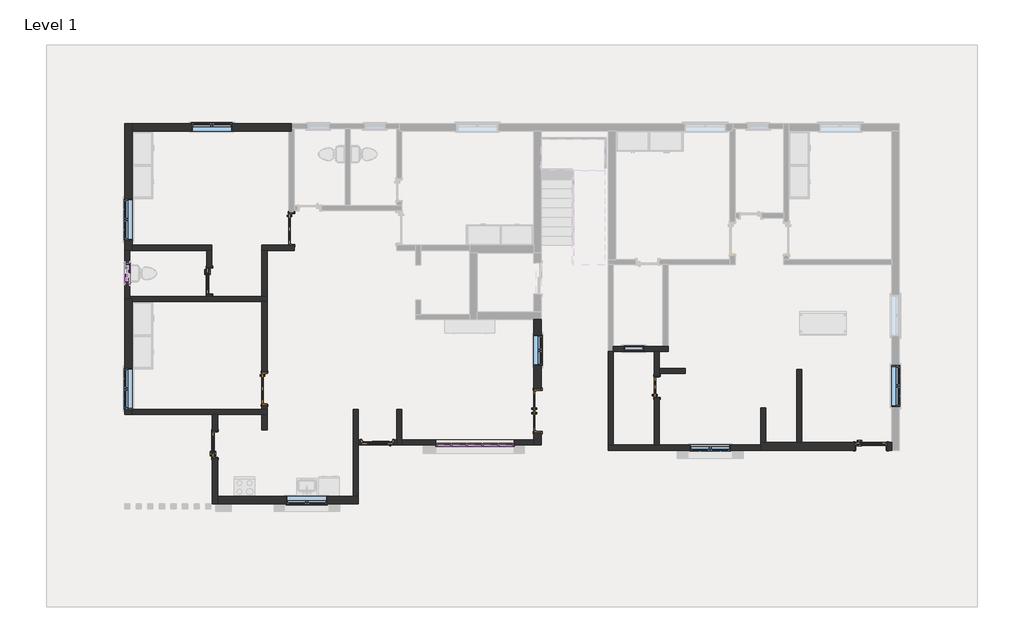
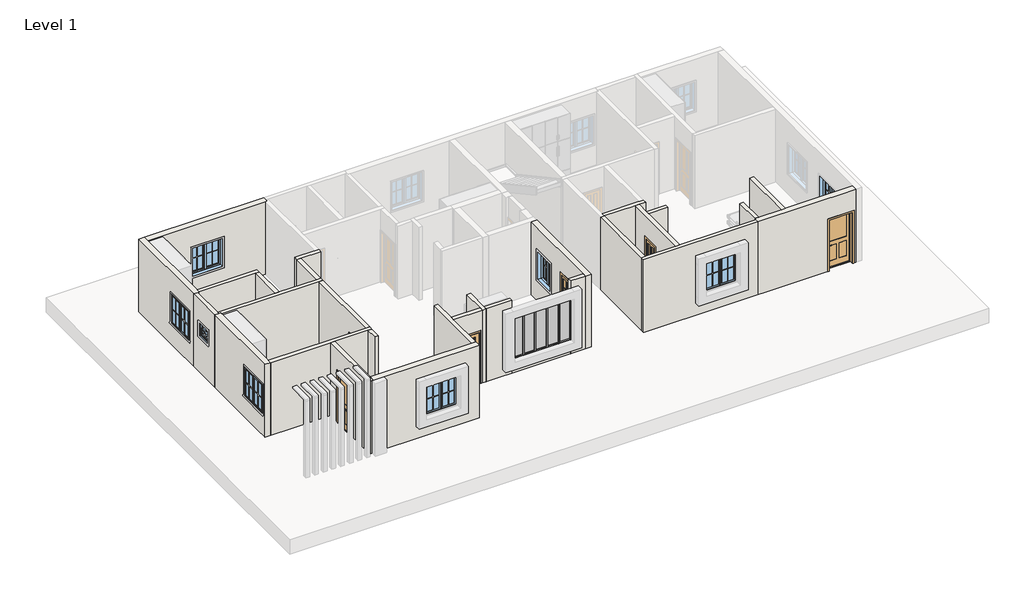
# One storey, part 1 of 3: 29 walls, 16 members, 9 windows, 8 doors, 5 plates.
# Revit data of these elements (continued)
# Elements 53, 54, 55, 56, 57, 58 (IfcWall, "9\"") (continued)
#   Top Constraint = Level 2
#   Materials on its faces: "wall"
# Element 59 (IfcWindow, "Window-Casement-Double : 3' X 4'")
#   Mark = "8"
#   Window Inset = 0' - 0"
#   Interior Wall Closure = 0' - 2 1/4"
#   Frame Extension = 0' - 0 1/4"
#   Exterior Wall Closure = 0' - 1 1/4"
#   Interior Trim Visibility = yes
#   Exterior Trim Visibility = yes
#   Phase Created = New Construction
#   Materials on its faces: "Wood - Stained", "Glass", "Clad - White"
# Element 60 (IfcWindow, "Window-Casement-Double : 4' X 4'")
#   Mark = "1"
#   Window Inset = 0' - 0"
#   Interior Wall Closure = 0' - 2 1/4"
#   Frame Extension = 0' - 0 1/4"
#   Exterior Wall Closure = 0' - 1 1/4"
#   Interior Trim Visibility = yes
#   Exterior Trim Visibility = yes
#   Phase Created = New Construction
#   Materials on its faces: "Wood - Stained", "Glass", "Clad - White"
# Element 61 (IfcWindow, "Window-Casement-Double : 4' X 4'")
#   Mark = "6"
#   Window Inset = 0' - 0"
#   Interior Wall Closure = 0' - 2 1/4"
#   Frame Extension = 0' - 0 1/4"
#   Exterior Wall Closure = 0' - 1 1/4"
#   Interior Trim Visibility = yes
#   Exterior Trim Visibility = yes
#   Phase Created = New Construction
#   Materials on its faces: "Wood - Stained", "Glass", "Clad - White"
# Element 62 (IfcWindow, "Window-Casement-Double : 4' X 4'")
#   Mark = "7"
#   Window Inset = 0' - 0"
#   Interior Wall Closure = 0' - 2 1/4"
#   Frame Extension = 0' - 0 1/4"
#   Exterior Wall Closure = 0' - 1 1/4"
#   Interior Trim Visibility = yes
#   Exterior Trim Visibility = yes
#   Phase Created = New Construction
#   Materials on its faces: "Wood - Stained", "Glass", "Clad - White"
# Element 63 (IfcWindow, "Window-Casement-Double : 4' X 4'")
#   Mark = "16"
#   Window Inset = 0' - 0"
#   Interior Wall Closure = 0' - 2 1/4"
#   Frame Extension = 0' - 0 1/4"
#   Exterior Wall Closure = 0' - 1 1/4"
#   Interior Trim Visibility = yes
#   Exterior Trim Visibility = yes
#   Phase Created = New Construction
#   Materials on its faces: "Wood - Stained", "Glass", "Clad - White"
# Element 64 (IfcWindow, "Window-Casement-Double : 4' X 4'")
#   Mark = "17"
#   Window Inset = 0' - 0"
#   Interior Wall Closure = 0' - 2 1/4"
#   Frame Extension = 0' - 0 1/4"
#   Exterior Wall Closure = 0' - 1 1/4"
#   Interior Trim Visibility = yes
#   Exterior Trim Visibility = yes
#   Phase Created = New Construction
#   Materials on its faces: "Wood - Stained", "Glass", "Clad - White"
# Element 65 (IfcWindow, "Window-Casement-Double : 4' X 4'")
#   Mark = "15"
#   Window Inset = 0' - 0"
#   Interior Wall Closure = 0' - 2 1/4"
#   Frame Extension = 0' - 0 1/4"
#   Exterior Wall Closure = 0' - 1 1/4"
#   Interior Trim Visibility = yes
#   Exterior Trim Visibility = yes
#   Phase Created = New Construction
#   Materials on its faces: "Wood - Stained", "Glass", "Clad - White"
# Element 66 (IfcWindow, "Window-Double-Hung : 2' X 2'")
#   Mark = "10"
#   Window Inset = 0' - 0"
#   Interior Wall Closure = 0' - 1 1/2"
#   Frame Extension = 0' - 1 1/4"
#   Exterior Wall Closure = 0' - 0 1/2"
#   Interior Trim Visibility = yes
#   Indicator Visibility = yes
#   Exterior Trim Visibility = yes
#   Phase Created = New Construction
#   Materials on its faces: "Wood - Stained", "Glass", "Clad - White"
# Element 67 (IfcWindow, "Window-Double-Hung : 2' X 2'")
#   Mark = "14"
#   Window Inset = 0' - 0"
#   Interior Wall Closure = 0' - 1 1/2"
#   Frame Extension = 0' - 1 1/4"
#   Exterior Wall Closure = 0' - 0 1/2"
#   Interior Trim Visibility = yes
#   Indicator Visibility = yes
#   Exterior Trim Visibility = yes
#   Phase Created = New Construction
#   Materials on its faces: "Wood - Stained", "Glass", "Clad - White"
# Materials
#   "Cherry": class "Wood", colour RGB 226 177 128, transparency 0, Description = "Prunus Serotina", Cost = 0
#   "Glass": class "Glass", colour RGB 0 128 192, transparency 0.75, Description = "Soda Lime Glass", Cost = 0
#   "Aluminum": class "Metal", colour RGB 247 247 247, transparency 0, Description = "Aluminum 6061", Cost = 0
#   "Metal - Stainless Steel": class "Metal", colour RGB 247 247 247, transparency 0
#   "Metal - Painted - Grey": class "Paint", colour RGB 104 104 104, transparency 0
#   "wall": class "Generic", colour RGB 127 127 127, transparency 0, Cost = 0
#   "Wood - Stained": class "Wood", colour RGB 224 178 126, transparency 0, Cost = 0
#   "Clad - White": class "Wood", colour RGB 242 242 238, transparency 0, Cost = 0
#   "exterior wall": class "Generic", colour RGB 215 217 121, transparency 0, Cost = 0
